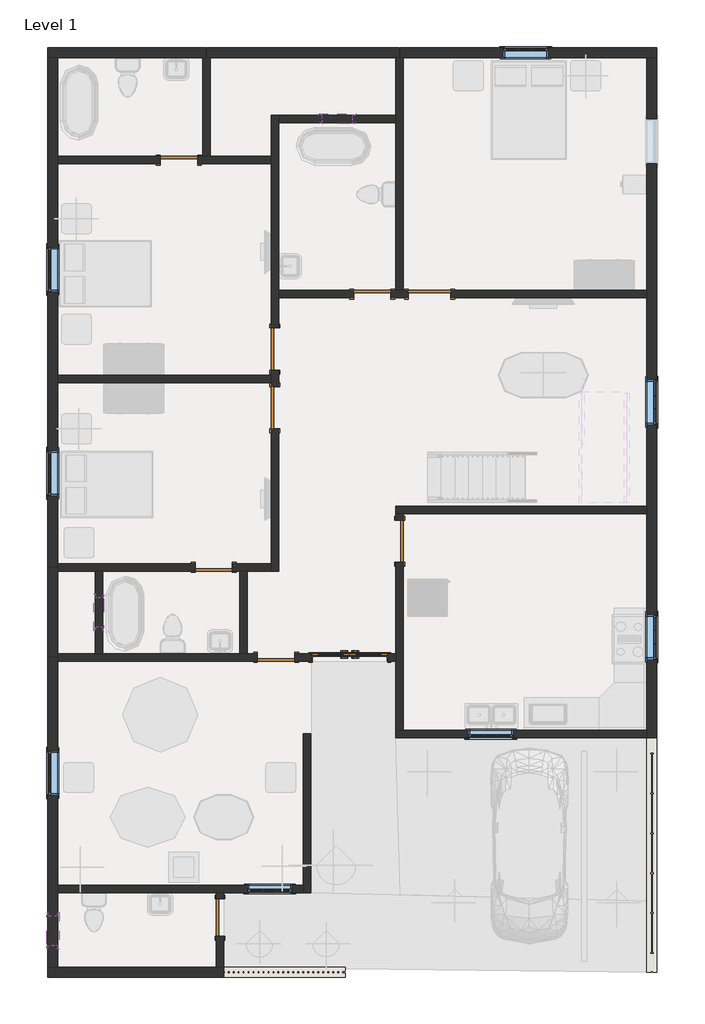
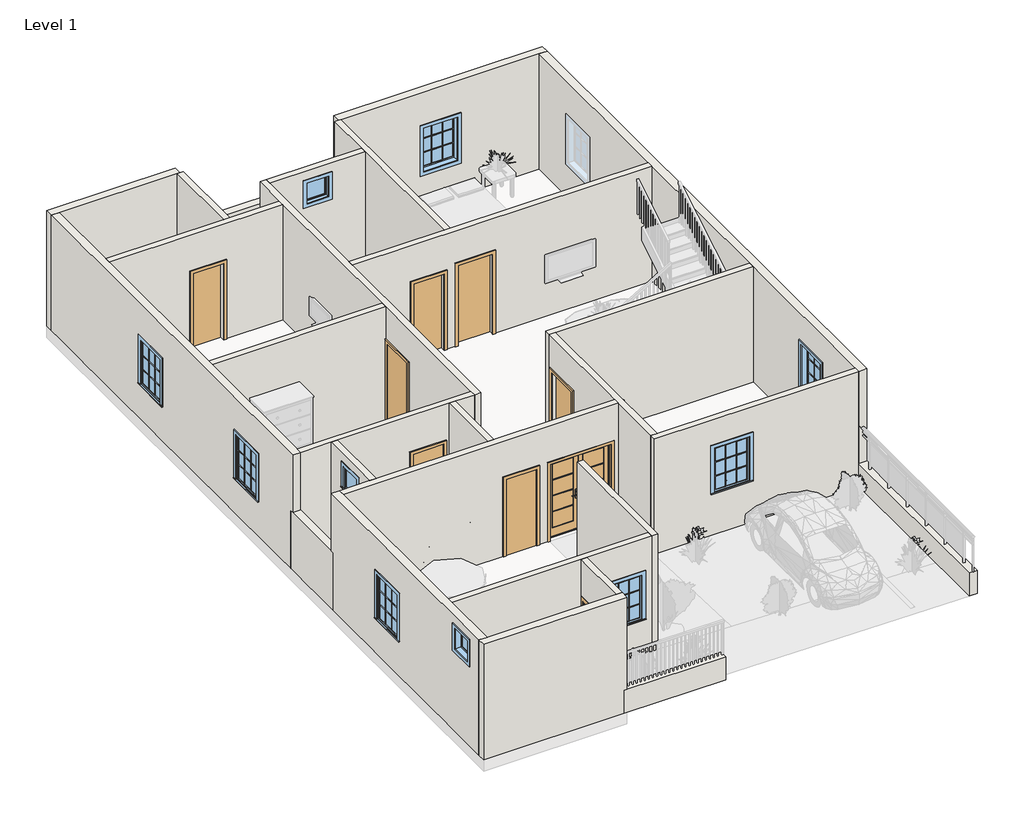
# One storey, part 1 of 3: 27 walls, 11 windows, 10 doors.
"""IFC4 building model written with IfcOpenShell, lengths in millimetres."""

from ifc_helpers import new_model, si_unit, frame, origin, origin_with_axes, place, context, project, spatial, polyline, outline, extrude, faceted_brep, transform, mapped, element, save
from components import door_94998e6c, door_255cab33, door_059fdd7e, door_99d96fc5, door_b6e9fca3, window_29c06734, window_5c190c7e, window_7947f0f9, window_e41d21a6, window_3d781103

model = new_model("IFC4")

# Units and contexts
model_context = context("Model", 3, world=origin())
ifc_project = project(units=[si_unit("LENGTHUNIT", "METRE", prefix="MILLI")], contexts=[model_context])

# Site, building, storey
site = spatial("IfcSite", under=ifc_project)
building = spatial("IfcBuilding", under=site)
storey = spatial("IfcBuildingStorey", under=building, Name="Level 1", Elevation=0.0)

# Doors
placement = place(None, origin())
door_shape = door_94998e6c(model_context)
element("IfcDoor", 1, ObjectType="Door-Exterior-Double-Full Glass-Wood_Clad : 60\" x 80\"", at=placement, inside=storey, context=model_context, shape_type="MappedRepresentation", body=[
    mapped(door_shape, transform((-5987.4789517, -1208.045591, 0.0), x_axis=(1.0, 0.0, 0.0), y_axis=(0.0, 1.0, 0.0), z_axis=(0.0, 0.0, 1.0))),
])
door_2_shape = door_255cab33(model_context)
element("IfcDoor", 2, ObjectType="Single-Flush : 30\" x 80\"", at=placement, inside=storey, context=model_context, shape_type="MappedRepresentation", body=[
    mapped(door_2_shape, transform((-8756.0789517, 617.579409, 0.0), x_axis=(1.0, 0.0, 0.0), y_axis=(0.0, 1.0, 0.0), z_axis=(0.0, 0.0, 1.0))),
])
element("IfcDoor", 3, ObjectType="Single-Flush : 30\" x 80\"", at=placement, inside=storey, context=model_context, shape_type="MappedRepresentation", body=[
    mapped(door_2_shape, transform((-7486.0789517, -1211.220591, 0.0), x_axis=(1.0, 0.0, 0.0), y_axis=(0.0, 1.0, 0.0), z_axis=(0.0, 0.0, 1.0))),
])
door_3_shape = door_059fdd7e(model_context)
element("IfcDoor", 4, ObjectType="Single-Flush : 30\" x 80\"", at=placement, inside=storey, context=model_context, shape_type="MappedRepresentation", body=[
    mapped(door_3_shape, transform((-9467.2789517, 8909.7768478, 0.0), x_axis=(1.0, 0.0, 0.0), y_axis=(0.0, 1.0, 0.0), z_axis=(0.0, 0.0, 1.0))),
])
element("IfcDoor", 5, ObjectType="Single-Flush : 30\" x 80\"", at=placement, inside=storey, context=model_context, shape_type="MappedRepresentation", body=[
    mapped(door_3_shape, transform((-5530.2789517, 6180.179409, 0.0), x_axis=(1.0, 0.0, 0.0), y_axis=(0.0, 1.0, 0.0), z_axis=(0.0, 0.0, 1.0))),
])
element("IfcDoor", 6, ObjectType="Single-Flush : 30\" x 80\"", at=placement, inside=storey, context=model_context, shape_type="MappedRepresentation", body=[
    mapped(door_3_shape, transform((-8629.0789517, -6508.0231522, 0.0), x_axis=(0.0, 1.0, 0.0), y_axis=(-1.0, 0.0, 0.0), z_axis=(0.0, 0.0, 1.0))),
])
door_4_shape = door_99d96fc5(model_context)
element("IfcDoor", 7, ObjectType="Single-Flush : 34\" x 84\"", at=placement, inside=storey, context=model_context, shape_type="MappedRepresentation", body=[
    mapped(door_4_shape, transform((-7511.4789517, 5062.579409, 0.0), x_axis=(0.0, -1.0, 0.0), y_axis=(1.0, 0.0, 0.0), z_axis=(0.0, 0.0, 1.0))),
])
element("IfcDoor", 8, ObjectType="Single-Flush : 34\" x 84\"", at=placement, inside=storey, context=model_context, shape_type="MappedRepresentation", body=[
    mapped(door_4_shape, transform((-4971.4789517, 1150.979409, 0.0), x_axis=(0.0, 1.0, 0.0), y_axis=(-1.0, 0.0, 0.0), z_axis=(0.0, 0.0, 1.0))),
])
element("IfcDoor", 9, ObjectType="Single-Flush : 34\" x 84\"", at=placement, inside=storey, context=model_context, shape_type="MappedRepresentation", body=[
    mapped(door_4_shape, transform((-4361.8789517, 6180.179409, 0.0), x_axis=(-1.0, 0.0, 0.0), y_axis=(0.0, -1.0, 0.0), z_axis=(0.0, 0.0, 1.0))),
])
door_5_shape = door_b6e9fca3(model_context)
element("IfcDoor", 10, ObjectType="Single-Flush : 34\" x 84\"", at=placement, inside=storey, context=model_context, shape_type="MappedRepresentation", body=[
    mapped(door_5_shape, transform((-7511.4789517, 3868.779409, 0.0), x_axis=(0.0, 1.0, 0.0), y_axis=(-1.0, 0.0, 0.0), z_axis=(0.0, 0.0, 1.0))),
])

# Walls
element("IfcWall", 11, ObjectType="Generic - 2'", at=placement, inside=storey, context=model_context, shape_type="Brep", body=[
    faceted_brep([(-6079.5539517, -7524.0231522, 0.0), (-8552.8789517, -7524.0231522, 0.0), (-8629.0789517, -7524.0231522, 0.0), (-8629.0789517, -7524.0231522, 609.6), (-6079.5539517, -7524.0231522, 609.6), (-6079.5539517, -7727.2231522, 0.0), (-6079.5539517, -7727.2231522, 609.6), (-8629.0789517, -7727.2231522, 609.6), (-8629.0789517, -7727.2231522, 0.0)], [[[0, 1, 2, 3, 4]], [[5, 6, 7, 8]], [[2, 1, 0, 5, 8]], [[3, 2, 8, 7]], [[4, 3, 7, 6]], [[0, 4, 6, 5]]]),
])
element("IfcWall", 12, ObjectType="Generic - 2'", at=placement, inside=storey, context=model_context, shape_type="Brep", body=[
    faceted_brep([(57.7210483, -2774.2231522, 0.0), (57.7210483, -2850.4231522, 0.0), (57.7210483, -7625.6231522, 0.0), (57.7210483, -7625.6231522, 609.6), (57.7210483, -2774.2231522, 609.6), (260.9210483, -2774.2231522, 0.0), (260.9210483, -2774.2231522, 609.6), (260.9210483, -7625.6231522, 609.6), (260.9210483, -7625.6231522, 0.0)], [[[0, 1, 2, 3, 4]], [[5, 6, 7, 8]], [[2, 1, 0, 5, 8]], [[3, 2, 8, 7]], [[4, 3, 7, 6]], [[0, 4, 6, 5]]]),
])
element("IfcWall", 13, ObjectType="Generic - 8\"", at=placement, inside=storey, context=model_context, shape_type="Brep", body=[
    faceted_brep([(-12134.2789517, 10992.5768478, 0.0), (-11931.0789517, 10992.5768478, 0.0), (-8921.1789517, 10992.5768478, 0.0), (-8921.1789517, 10992.5768478, 3048.0), (-11931.0789517, 10992.5768478, 3048.0), (-12134.2789517, 10992.5768478, 3048.0), (-12134.2789517, 11195.7768478, 0.0), (-12134.2789517, 11195.7768478, 3048.0), (-8921.1789517, 11195.7768478, 3048.0), (-8921.1789517, 11195.7768478, 0.0)], [[[0, 1, 2, 3, 4, 5]], [[6, 7, 8, 9]], [[2, 1, 0, 6, 9]], [[3, 2, 9, 8]], [[0, 5, 7, 6]], [[5, 4, 3, 8, 7]]]),
])
element("IfcWall", 14, ObjectType="Generic - 8\"", at=placement, inside=storey, context=model_context, shape_type="Brep", body=[
    faceted_brep([(57.7210483, 10992.5768478, 0.0), (57.7210483, 6256.379409, 0.0), (57.7210483, 6103.979409, 0.0), (57.7210483, 1862.179409, 0.0), (57.7210483, 1709.779409, 0.0), (57.7210483, -2698.0231522, 0.0), (57.7210483, -2774.2231522, 0.0), (57.7210483, -2774.2231522, 609.6), (57.7210483, -2850.4231522, 609.6), (57.7210483, -2850.4231522, 3048.0), (57.7210483, -2698.0231522, 3048.0), (57.7210483, 1709.779409, 3048.0), (57.7210483, 1862.179409, 3048.0), (57.7210483, 6103.979409, 3048.0), (57.7210483, 6256.379409, 3048.0), (57.7210483, 10992.5768478, 3048.0), (57.7210483, -1256.1218716, 2286.0), (57.7210483, -1256.1218716, 1066.8), (57.7210483, -341.7218716, 1066.8), (57.7210483, -341.7218716, 2286.0), (57.7210483, 3525.879409, 2133.6), (57.7210483, 3525.879409, 914.4), (57.7210483, 4440.279409, 914.4), (57.7210483, 4440.279409, 2133.6), (57.7210483, 8833.5768478, 2133.6), (57.7210483, 8833.5768478, 914.4), (57.7210483, 9747.9768478, 914.4), (57.7210483, 9747.9768478, 2133.6), (260.9210483, 10992.5768478, 0.0), (260.9210483, 10992.5768478, 3048.0), (260.9210483, -2850.4231522, 3048.0), (260.9210483, -2850.4231522, 609.6), (260.9210483, -2774.2231522, 609.6), (260.9210483, -2774.2231522, 0.0), (260.9210483, -1256.1218716, 2286.0), (260.9210483, -341.7218716, 2286.0), (260.9210483, -341.7218716, 1066.8), (260.9210483, -1256.1218716, 1066.8), (260.9210483, 3525.879409, 2133.6), (260.9210483, 4440.279409, 2133.6), (260.9210483, 4440.279409, 914.4), (260.9210483, 3525.879409, 914.4), (260.9210483, 8833.5768478, 2133.6), (260.9210483, 9747.9768478, 2133.6), (260.9210483, 9747.9768478, 914.4), (260.9210483, 8833.5768478, 914.4)], [[[0, 1, 2, 3, 4, 5, 6, 7, 8, 9, 10, 11, 12, 13, 14, 15], [16, 17, 18, 19], [20, 21, 22, 23], [24, 25, 26, 27]], [[28, 29, 30, 31, 32, 33], [34, 35, 36, 37], [38, 39, 40, 41], [42, 43, 44, 45]], [[6, 5, 4, 3, 2, 1, 0, 28, 33]], [[0, 15, 29, 28]], [[17, 16, 34, 37]], [[18, 17, 37, 36]], [[19, 18, 36, 35]], [[16, 19, 35, 34]], [[21, 20, 38, 41]], [[22, 21, 41, 40]], [[23, 22, 40, 39]], [[20, 23, 39, 38]], [[25, 24, 42, 45]], [[26, 25, 45, 44]], [[27, 26, 44, 43]], [[24, 27, 43, 42]], [[7, 6, 33, 32]], [[31, 8, 7, 32]], [[9, 8, 31, 30]], [[15, 14, 13, 12, 11, 10, 9, 30, 29]]]),
])
element("IfcWall", 15, ObjectType="Generic - 8\"", at=placement, inside=storey, context=model_context, shape_type="Brep", body=[
    faceted_brep([(-11931.0789517, -7524.0231522, 0.0), (-11931.0789517, -6000.0231522, 0.0), (-11931.0789517, -5847.6231522, 0.0), (-11931.0789517, -1287.420591, 0.0), (-11931.0789517, -1211.220591, 0.0), (-11931.0789517, -1211.220591, 1524.0), (-11931.0789517, -1135.020591, 1524.0), (-11931.0789517, -1135.020591, 3048.0), (-11931.0789517, -1287.420591, 3048.0), (-11931.0789517, -5847.6231522, 3048.0), (-11931.0789517, -6000.0231522, 3048.0), (-11931.0789517, -7524.0231522, 3048.0), (-11931.0789517, -3110.3218716, 2133.6), (-11931.0789517, -3110.3218716, 914.4), (-11931.0789517, -4024.7218716, 914.4), (-11931.0789517, -4024.7218716, 2133.6), (-11931.0789517, -7079.5231522, 2768.6), (-11931.0789517, -6469.9231522, 2768.6), (-11931.0789517, -6469.9231522, 2159.0), (-11931.0789517, -7079.5231522, 2159.0), (-12134.2789517, -7524.0231522, 0.0), (-12134.2789517, -7524.0231522, 3048.0), (-12134.2789517, -1135.020591, 3048.0), (-12134.2789517, -1135.020591, 1524.0), (-12134.2789517, -1211.220591, 1524.0), (-12134.2789517, -1211.220591, 0.0), (-12134.2789517, -3110.3218716, 2133.6), (-12134.2789517, -4024.7218716, 2133.6), (-12134.2789517, -4024.7218716, 914.4), (-12134.2789517, -3110.3218716, 914.4), (-12134.2789517, -7079.5231522, 2768.6), (-12134.2789517, -7079.5231522, 2159.0), (-12134.2789517, -6469.9231522, 2159.0), (-12134.2789517, -6469.9231522, 2768.6)], [[[0, 1, 2, 3, 4, 5, 6, 7, 8, 9, 10, 11], [12, 13, 14, 15], [16, 17, 18, 19]], [[20, 21, 22, 23, 24, 25], [26, 27, 28, 29], [30, 31, 32, 33]], [[4, 3, 2, 1, 0, 20, 25]], [[0, 11, 21, 20]], [[13, 12, 26, 29]], [[14, 13, 29, 28]], [[15, 14, 28, 27]], [[12, 15, 27, 26]], [[31, 30, 16, 19]], [[32, 31, 19, 18]], [[33, 32, 18, 17]], [[30, 33, 17, 16]], [[5, 4, 25, 24]], [[23, 6, 5, 24]], [[7, 6, 23, 22]], [[11, 10, 9, 8, 7, 22, 21]]]),
])
element("IfcWall", 16, ObjectType="Generic - 8\"", at=placement, inside=storey, context=model_context, shape_type="Brep", body=[
    faceted_brep([(-8629.0789517, -7524.0231522, 0.0), (-8705.2789517, -7524.0231522, 0.0), (-11931.0789517, -7524.0231522, 0.0), (-12134.2789517, -7524.0231522, 0.0), (-12134.2789517, -7524.0231522, 3048.0), (-11931.0789517, -7524.0231522, 3048.0), (-8705.2789517, -7524.0231522, 3048.0), (-8552.8789517, -7524.0231522, 3048.0), (-8552.8789517, -7524.0231522, 609.6), (-8629.0789517, -7524.0231522, 609.6), (-8629.0789517, -7727.2231522, 0.0), (-8629.0789517, -7727.2231522, 609.6), (-8552.8789517, -7727.2231522, 609.6), (-8552.8789517, -7727.2231522, 3048.0), (-12134.2789517, -7727.2231522, 3048.0), (-12134.2789517, -7727.2231522, 0.0)], [[[0, 1, 2, 3, 4, 5, 6, 7, 8, 9]], [[10, 11, 12, 13, 14, 15]], [[3, 2, 1, 0, 10, 15]], [[4, 3, 15, 14]], [[0, 9, 11, 10]], [[8, 12, 11, 9]], [[8, 7, 13, 12]], [[7, 6, 5, 4, 14, 13]]]),
])
element("IfcWall", 17, ObjectType="Generic - 8\"", at=placement, inside=storey, context=model_context, shape_type="Brep", body=[
    faceted_brep([(-8895.7789517, 10992.5768478, 0.0), (-8832.2789517, 10992.5768478, 0.0), (-4984.1789517, 10992.5768478, 0.0), (-4984.1789517, 10992.5768478, 1524.0), (-8895.7789517, 10992.5768478, 1524.0), (-8895.7789517, 11195.7768478, 0.0), (-8895.7789517, 11195.7768478, 1524.0), (-4984.1789517, 11195.7768478, 1524.0), (-4984.1789517, 11195.7768478, 0.0)], [[[0, 1, 2, 3, 4]], [[5, 6, 7, 8]], [[2, 1, 0, 5, 8]], [[3, 2, 8, 7]], [[4, 3, 7, 6]], [[0, 4, 6, 5]]]),
])
element("IfcWall", 18, ObjectType="Generic - 8\"", at=placement, inside=storey, context=model_context, shape_type="Brep", body=[
    faceted_brep([(-4958.7789517, 10992.5768478, 0.0), (-4895.2789517, 10992.5768478, 0.0), (57.7210483, 10992.5768478, 0.0), (260.9210483, 10992.5768478, 0.0), (260.9210483, 10992.5768478, 3048.0), (57.7210483, 10992.5768478, 3048.0), (-4895.2789517, 10992.5768478, 3048.0), (-4958.7789517, 10992.5768478, 3048.0), (-1948.8789517, 10992.5768478, 2133.6), (-1948.8789517, 10992.5768478, 914.4), (-2863.2789517, 10992.5768478, 914.4), (-2863.2789517, 10992.5768478, 2133.6), (-4958.7789517, 11195.7768478, 0.0), (-4958.7789517, 11195.7768478, 3048.0), (260.9210483, 11195.7768478, 3048.0), (260.9210483, 11195.7768478, 0.0), (-1948.8789517, 11195.7768478, 2133.6), (-2863.2789517, 11195.7768478, 2133.6), (-2863.2789517, 11195.7768478, 914.4), (-1948.8789517, 11195.7768478, 914.4)], [[[0, 1, 2, 3, 4, 5, 6, 7], [8, 9, 10, 11]], [[12, 13, 14, 15], [16, 17, 18, 19]], [[3, 2, 1, 0, 12, 15]], [[0, 7, 13, 12]], [[4, 3, 15, 14]], [[8, 11, 17, 16]], [[11, 10, 18, 17]], [[10, 9, 19, 18]], [[9, 8, 16, 19]], [[7, 6, 5, 4, 14, 13]]]),
])
element("IfcWall", 19, ObjectType="Generic - 8\"", at=placement, inside=storey, context=model_context, shape_type="Brep", body=[
    faceted_brep([(-11931.0789517, 617.579409, 0.0), (-11931.0789517, 693.779409, 0.0), (-11931.0789517, 4376.779409, 0.0), (-11931.0789517, 4529.179409, 0.0), (-11931.0789517, 8833.5768478, 0.0), (-11931.0789517, 8985.9768478, 0.0), (-11931.0789517, 10992.5768478, 0.0), (-11931.0789517, 10992.5768478, 3048.0), (-11931.0789517, 8985.9768478, 3048.0), (-11931.0789517, 8833.5768478, 3048.0), (-11931.0789517, 4529.179409, 3048.0), (-11931.0789517, 4376.779409, 3048.0), (-11931.0789517, 693.779409, 3048.0), (-11931.0789517, 541.379409, 3048.0), (-11931.0789517, 541.379409, 1524.0), (-11931.0789517, 617.579409, 1524.0), (-11931.0789517, 7138.5781284, 2133.6), (-11931.0789517, 7138.5781284, 914.4), (-11931.0789517, 6224.1781284, 914.4), (-11931.0789517, 6224.1781284, 2133.6), (-11931.0789517, 2992.479409, 2133.6), (-11931.0789517, 2992.479409, 914.4), (-11931.0789517, 2078.079409, 914.4), (-11931.0789517, 2078.079409, 2133.6), (-12134.2789517, 617.579409, 0.0), (-12134.2789517, 617.579409, 1524.0), (-12134.2789517, 541.379409, 1524.0), (-12134.2789517, 541.379409, 3048.0), (-12134.2789517, 10992.5768478, 3048.0), (-12134.2789517, 10992.5768478, 0.0), (-12134.2789517, 7138.5781284, 2133.6), (-12134.2789517, 6224.1781284, 2133.6), (-12134.2789517, 6224.1781284, 914.4), (-12134.2789517, 7138.5781284, 914.4), (-12134.2789517, 2992.479409, 2133.6), (-12134.2789517, 2078.079409, 2133.6), (-12134.2789517, 2078.079409, 914.4), (-12134.2789517, 2992.479409, 914.4)], [[[0, 1, 2, 3, 4, 5, 6, 7, 8, 9, 10, 11, 12, 13, 14, 15], [16, 17, 18, 19], [20, 21, 22, 23]], [[24, 25, 26, 27, 28, 29], [30, 31, 32, 33], [34, 35, 36, 37]], [[6, 5, 4, 3, 2, 1, 0, 24, 29]], [[7, 6, 29, 28]], [[16, 19, 31, 30]], [[19, 18, 32, 31]], [[18, 17, 33, 32]], [[17, 16, 30, 33]], [[20, 23, 35, 34]], [[23, 22, 36, 35]], [[22, 21, 37, 36]], [[21, 20, 34, 37]], [[0, 15, 25, 24]], [[14, 26, 25, 15]], [[14, 13, 27, 26]], [[13, 12, 11, 10, 9, 8, 7, 28, 27]]]),
])
element("IfcWall", 20, ObjectType="Generic - 8\"", at=placement, inside=storey, context=model_context, shape_type="Brep", body=[
    faceted_brep([(-11931.0789517, -1211.220591, 0.0), (-11931.0789517, -1135.020591, 0.0), (-11931.0789517, 541.379409, 0.0), (-11931.0789517, 617.579409, 0.0), (-11931.0789517, 617.579409, 1524.0), (-11931.0789517, 541.379409, 1524.0), (-11931.0789517, -1135.020591, 1524.0), (-11931.0789517, -1211.220591, 1524.0), (-12134.2789517, -1211.220591, 0.0), (-12134.2789517, -1211.220591, 1524.0), (-12134.2789517, -1135.020591, 1524.0), (-12134.2789517, 541.379409, 1524.0), (-12134.2789517, 617.579409, 1524.0), (-12134.2789517, 617.579409, 0.0)], [[[0, 1, 2, 3, 4, 5, 6, 7]], [[8, 9, 10, 11, 12, 13]], [[3, 2, 1, 0, 8, 13]], [[4, 3, 13, 12]], [[7, 6, 5, 4, 12, 11, 10, 9]], [[0, 7, 9, 8]]]),
])
element("IfcWall", 21, ObjectType="INNER 6\"", at=placement, inside=storey, context=model_context, shape_type="Brep", body=[
    faceted_brep([(-9086.2789517, 8833.5768478, 2032.0), (-9086.2789517, 8833.5768478, 0.0), (-7587.6789517, 8833.5768478, 0.0), (-7587.6789517, 8833.5768478, 3048.0), (-11931.0789517, 8833.5768478, 3048.0), (-11931.0789517, 8833.5768478, 0.0), (-9848.2789517, 8833.5768478, 0.0), (-9848.2789517, 8833.5768478, 2032.0), (-7587.6789517, 8985.9768478, 0.0), (-8832.2789517, 8985.9768478, 0.0), (-8984.6789517, 8985.9768478, 0.0), (-9086.2789517, 8985.9768478, 0.0), (-9086.2789517, 8985.9768478, 2032.0), (-9848.2789517, 8985.9768478, 2032.0), (-9848.2789517, 8985.9768478, 0.0), (-11931.0789517, 8985.9768478, 0.0), (-11931.0789517, 8985.9768478, 3048.0), (-8984.6789517, 8985.9768478, 3048.0), (-8832.2789517, 8985.9768478, 3048.0), (-7587.6789517, 8985.9768478, 3048.0)], [[[0, 1, 2, 3, 4, 5, 6, 7]], [[8, 9, 10, 11, 12, 13, 14, 15, 16, 17, 18, 19]], [[6, 5, 15, 14]], [[2, 1, 11, 10, 9, 8]], [[5, 4, 16, 15]], [[3, 2, 8, 19]], [[12, 11, 1, 0]], [[13, 12, 0, 7]], [[14, 13, 7, 6]], [[4, 3, 19, 18, 17, 16]]]),
])
element("IfcWall", 22, ObjectType="INNER 6\"", at=placement, inside=storey, context=model_context, shape_type="Brep", body=[
    faceted_brep([(-8832.2789517, 8985.9768478, 0.0), (-8832.2789517, 10992.5768478, 0.0), (-8832.2789517, 10992.5768478, 3048.0), (-8832.2789517, 8985.9768478, 3048.0), (-8984.6789517, 8985.9768478, 0.0), (-8984.6789517, 8985.9768478, 3048.0), (-8984.6789517, 10992.5768478, 3048.0), (-8984.6789517, 10992.5768478, 0.0), (-8895.7789517, 10992.5768478, 0.0)], [[[0, 1, 2, 3]], [[4, 5, 6, 7]], [[1, 0, 4, 7, 8]], [[0, 3, 5, 4]], [[2, 1, 8, 7, 6]], [[3, 2, 6, 5]]]),
])
element("IfcWall", 23, ObjectType="INNER 6\"", at=placement, inside=storey, context=model_context, shape_type="Brep", body=[
    faceted_brep([(-7435.2789517, 4300.579409, 2133.6), (-7435.2789517, 4300.579409, 0.0), (-7435.2789517, 4630.779409, 0.0), (-7435.2789517, 4630.779409, 2133.6), (-7435.2789517, 5494.379409, 2133.6), (-7435.2789517, 5494.379409, 0.0), (-7435.2789517, 6103.979409, 0.0), (-7435.2789517, 6256.379409, 0.0), (-7435.2789517, 9671.7768478, 0.0), (-7435.2789517, 9824.1768478, 0.0), (-7435.2789517, 9824.1768478, 3048.0), (-7435.2789517, 9671.7768478, 3048.0), (-7435.2789517, 6256.379409, 3048.0), (-7435.2789517, 6103.979409, 3048.0), (-7435.2789517, 541.379409, 3048.0), (-7435.2789517, 541.379409, 0.0), (-7435.2789517, 3436.979409, 0.0), (-7435.2789517, 3436.979409, 2133.6), (-7587.6789517, 4630.779409, 0.0), (-7587.6789517, 4529.179409, 0.0), (-7587.6789517, 4376.779409, 0.0), (-7587.6789517, 4300.579409, 0.0), (-7587.6789517, 4300.579409, 2133.6), (-7587.6789517, 3436.979409, 2133.6), (-7587.6789517, 3436.979409, 0.0), (-7587.6789517, 693.779409, 0.0), (-7587.6789517, 541.379409, 0.0), (-7587.6789517, 541.379409, 3048.0), (-7587.6789517, 693.779409, 3048.0), (-7587.6789517, 4376.779409, 3048.0), (-7587.6789517, 4529.179409, 3048.0), (-7587.6789517, 8833.5768478, 3048.0), (-7587.6789517, 8985.9768478, 3048.0), (-7587.6789517, 9824.1768478, 3048.0), (-7587.6789517, 9824.1768478, 0.0), (-7587.6789517, 8985.9768478, 0.0), (-7587.6789517, 8833.5768478, 0.0), (-7587.6789517, 5494.379409, 0.0), (-7587.6789517, 5494.379409, 2133.6), (-7587.6789517, 4630.779409, 2133.6)], [[[0, 1, 2, 3, 4, 5, 6, 7, 8, 9, 10, 11, 12, 13, 14, 15, 16, 17]], [[18, 19, 20, 21, 22, 23, 24, 25, 26, 27, 28, 29, 30, 31, 32, 33, 34, 35, 36, 37, 38, 39]], [[37, 36, 35, 34, 9, 8, 7, 6, 5]], [[16, 15, 26, 25, 24]], [[2, 1, 21, 20, 19, 18]], [[10, 9, 34, 33]], [[15, 14, 27, 26]], [[3, 2, 18, 39]], [[4, 3, 39, 38]], [[5, 4, 38, 37]], [[22, 21, 1, 0]], [[23, 22, 0, 17]], [[24, 23, 17, 16]], [[14, 13, 12, 11, 10, 33, 32, 31, 30, 29, 28, 27]]]),
])
element("IfcWall", 24, ObjectType="INNER 6\"", at=placement, inside=storey, context=model_context, shape_type="SweptSolid", body=[
    extrude(outline(polyline([(0.0, -7435.2789517), (0.0, -5047.6789517), (3048.0, -5047.6789517), (3048.0, -7435.2789517), (0.0, -7435.2789517)]), holes=[polyline([(2768.6, -5936.6789517), (2159.0, -5936.6789517), (2159.0, -6546.2789517), (2768.6, -6546.2789517), (2768.6, -5936.6789517)])]), frame((0.0, 9671.7768478, 0.0), z_axis=(0.0, 1.0, 0.0), x_axis=(0.0, 0.0, 1.0)), (0.0, 0.0, 1.0), 152.4),
])
element("IfcWall", 25, ObjectType="INNER 6\"", at=placement, inside=storey, context=model_context, shape_type="Brep", body=[
    faceted_brep([(-5047.6789517, 10992.5768478, 0.0), (-5047.6789517, 9824.1768478, 0.0), (-5047.6789517, 9671.7768478, 0.0), (-5047.6789517, 6256.379409, 0.0), (-5047.6789517, 6256.379409, 3048.0), (-5047.6789517, 9671.7768478, 3048.0), (-5047.6789517, 9824.1768478, 3048.0), (-5047.6789517, 10992.5768478, 3048.0), (-4895.2789517, 10992.5768478, 0.0), (-4895.2789517, 10992.5768478, 3048.0), (-4895.2789517, 6256.379409, 3048.0), (-4895.2789517, 6256.379409, 0.0), (-4958.7789517, 10992.5768478, 0.0), (-4958.7789517, 10992.5768478, 3048.0)], [[[0, 1, 2, 3, 4, 5, 6, 7]], [[8, 9, 10, 11]], [[3, 2, 1, 0, 12, 8, 11]], [[0, 7, 13, 9, 8, 12]], [[4, 3, 11, 10]], [[7, 6, 5, 4, 10, 9, 13]]]),
])
element("IfcWall", 26, ObjectType="INNER 6\"", at=placement, inside=storey, context=model_context, shape_type="Brep", body=[
    faceted_brep([(-5149.2789517, 6103.979409, 2032.0), (-5149.2789517, 6103.979409, 0.0), (-4793.6789517, 6103.979409, 0.0), (-4793.6789517, 6103.979409, 2133.6), (-3930.0789517, 6103.979409, 2133.6), (-3930.0789517, 6103.979409, 0.0), (57.7210483, 6103.979409, 0.0), (57.7210483, 6103.979409, 3048.0), (-7435.2789517, 6103.979409, 3048.0), (-7435.2789517, 6103.979409, 0.0), (-5911.2789517, 6103.979409, 0.0), (-5911.2789517, 6103.979409, 2032.0), (-4793.6789517, 6256.379409, 0.0), (-4895.2789517, 6256.379409, 0.0), (-5047.6789517, 6256.379409, 0.0), (-5149.2789517, 6256.379409, 0.0), (-5149.2789517, 6256.379409, 2032.0), (-5911.2789517, 6256.379409, 2032.0), (-5911.2789517, 6256.379409, 0.0), (-7435.2789517, 6256.379409, 0.0), (-7435.2789517, 6256.379409, 3048.0), (-5047.6789517, 6256.379409, 3048.0), (-4895.2789517, 6256.379409, 3048.0), (57.7210483, 6256.379409, 3048.0), (57.7210483, 6256.379409, 0.0), (-3930.0789517, 6256.379409, 0.0), (-3930.0789517, 6256.379409, 2133.6), (-4793.6789517, 6256.379409, 2133.6)], [[[0, 1, 2, 3, 4, 5, 6, 7, 8, 9, 10, 11]], [[12, 13, 14, 15, 16, 17, 18, 19, 20, 21, 22, 23, 24, 25, 26, 27]], [[25, 24, 6, 5]], [[10, 9, 19, 18]], [[2, 1, 15, 14, 13, 12]], [[7, 6, 24, 23]], [[9, 8, 20, 19]], [[3, 2, 12, 27]], [[4, 3, 27, 26]], [[5, 4, 26, 25]], [[16, 15, 1, 0]], [[17, 16, 0, 11]], [[18, 17, 11, 10]], [[8, 7, 23, 22, 21, 20]]]),
])
element("IfcWall", 27, ObjectType="INNER 6\"", at=placement, inside=storey, context=model_context, shape_type="Brep", body=[
    faceted_brep([(-5047.6789517, 1709.779409, 0.0), (-4895.2789517, 1709.779409, 0.0), (57.7210483, 1709.779409, 0.0), (57.7210483, 1709.779409, 3048.0), (-4895.2789517, 1709.779409, 3048.0), (-5047.6789517, 1709.779409, 3048.0), (-5047.6789517, 1862.179409, 0.0), (-5047.6789517, 1862.179409, 3048.0), (57.7210483, 1862.179409, 3048.0), (57.7210483, 1862.179409, 0.0)], [[[0, 1, 2, 3, 4, 5]], [[6, 7, 8, 9]], [[2, 1, 0, 6, 9]], [[3, 2, 9, 8]], [[0, 5, 7, 6]], [[5, 4, 3, 8, 7]]]),
])
element("IfcWall", 28, ObjectType="INNER 6\"", at=placement, inside=storey, context=model_context, shape_type="Brep", body=[
    faceted_brep([(-5047.6789517, -2850.4231522, 0.0), (57.7210483, -2850.4231522, 0.0), (57.7210483, -2850.4231522, 609.6), (57.7210483, -2850.4231522, 3048.0), (-5047.6789517, -2850.4231522, 3048.0), (-3574.4789517, -2850.4231522, 2311.4), (-2660.0789517, -2850.4231522, 2311.4), (-2660.0789517, -2850.4231522, 1092.2), (-3574.4789517, -2850.4231522, 1092.2), (-5047.6789517, -2698.0231522, 0.0), (-5047.6789517, -2698.0231522, 3048.0), (-4895.2789517, -2698.0231522, 3048.0), (57.7210483, -2698.0231522, 3048.0), (57.7210483, -2698.0231522, 0.0), (-4895.2789517, -2698.0231522, 0.0), (-3574.4789517, -2698.0231522, 2311.4), (-3574.4789517, -2698.0231522, 1092.2), (-2660.0789517, -2698.0231522, 1092.2), (-2660.0789517, -2698.0231522, 2311.4), (57.7210483, -2774.2231522, 0.0)], [[[0, 1, 2, 3, 4], [5, 6, 7, 8]], [[9, 10, 11, 12, 13, 14], [15, 16, 17, 18]], [[1, 0, 9, 14, 13, 19]], [[0, 4, 10, 9]], [[16, 15, 5, 8]], [[17, 16, 8, 7]], [[18, 17, 7, 6]], [[15, 18, 6, 5]], [[1, 19, 13, 12, 3, 2]], [[4, 3, 12, 11, 10]]]),
])
element("IfcWall", 29, ObjectType="INNER 6\"", at=placement, inside=storey, context=model_context, shape_type="SweptSolid", body=[
    extrude(outline(polyline([(-7587.6789517, 4376.779409), (-11931.0789517, 4376.779409), (-11931.0789517, 4529.179409), (-7587.6789517, 4529.179409), (-7587.6789517, 4376.779409)])), origin_with_axes(), (0.0, 0.0, 1.0), 3048.0),
])
element("IfcWall", 30, ObjectType="INNER 6\"", at=placement, inside=storey, context=model_context, shape_type="Brep", body=[
    faceted_brep([(-7587.6789517, 693.779409, 0.0), (-8375.0789517, 693.779409, 0.0), (-8375.0789517, 693.779409, 2032.0), (-9137.0789517, 693.779409, 2032.0), (-9137.0789517, 693.779409, 0.0), (-11931.0789517, 693.779409, 0.0), (-11931.0789517, 693.779409, 3048.0), (-7587.6789517, 693.779409, 3048.0), (-8375.0789517, 541.379409, 2032.0), (-8375.0789517, 541.379409, 0.0), (-8222.6789517, 541.379409, 0.0), (-8070.2789517, 541.379409, 0.0), (-7587.6789517, 541.379409, 0.0), (-7587.6789517, 541.379409, 3048.0), (-8070.2789517, 541.379409, 3048.0), (-8222.6789517, 541.379409, 3048.0), (-11016.6789517, 541.379409, 3048.0), (-11169.0789517, 541.379409, 3048.0), (-11931.0789517, 541.379409, 3048.0), (-11931.0789517, 541.379409, 1524.0), (-11931.0789517, 541.379409, 0.0), (-11169.0789517, 541.379409, 0.0), (-11016.6789517, 541.379409, 0.0), (-9137.0789517, 541.379409, 0.0), (-9137.0789517, 541.379409, 2032.0), (-11931.0789517, 617.579409, 0.0)], [[[0, 1, 2, 3, 4, 5, 6, 7]], [[8, 9, 10, 11, 12, 13, 14, 15, 16, 17, 18, 19, 20, 21, 22, 23, 24]], [[12, 11, 10, 9, 1, 0]], [[23, 22, 21, 20, 25, 5, 4]], [[0, 7, 13, 12]], [[2, 1, 9, 8]], [[3, 2, 8, 24]], [[4, 3, 24, 23]], [[5, 25, 20, 19, 18, 6]], [[7, 6, 18, 17, 16, 15, 14, 13]]]),
])
element("IfcWall", 31, ObjectType="INNER 6\"", at=placement, inside=storey, context=model_context, shape_type="SweptSolid", body=[
    extrude(outline(polyline([(-8222.6789517, -1135.020591), (-8222.6789517, 541.379409), (-8070.2789517, 541.379409), (-8070.2789517, -1135.020591), (-8222.6789517, -1135.020591)])), origin_with_axes(), (0.0, 0.0, 1.0), 3048.0),
])
element("IfcWall", 32, ObjectType="INNER 6\"", at=placement, inside=storey, context=model_context, shape_type="Brep", body=[
    faceted_brep([(-5047.6789517, -1135.020591, 3048.0), (-5047.6789517, -1135.020591, 0.0), (-5200.0789517, -1135.020591, 0.0), (-5200.0789517, -1135.020591, 2057.4), (-6774.8789517, -1135.020591, 2057.4), (-6774.8789517, -1135.020591, 0.0), (-7105.0789517, -1135.020591, 0.0), (-7105.0789517, -1135.020591, 2032.0), (-7867.0789517, -1135.020591, 2032.0), (-7867.0789517, -1135.020591, 0.0), (-8070.2789517, -1135.020591, 0.0), (-8222.6789517, -1135.020591, 0.0), (-11016.6789517, -1135.020591, 0.0), (-11169.0789517, -1135.020591, 0.0), (-11931.0789517, -1135.020591, 0.0), (-11931.0789517, -1135.020591, 1524.0), (-11931.0789517, -1135.020591, 3048.0), (-11169.0789517, -1135.020591, 3048.0), (-11016.6789517, -1135.020591, 3048.0), (-8222.6789517, -1135.020591, 3048.0), (-8070.2789517, -1135.020591, 3048.0), (-5047.6789517, -1287.420591, 0.0), (-5047.6789517, -1287.420591, 3048.0), (-6774.8789517, -1287.420591, 3048.0), (-11931.0789517, -1287.420591, 3048.0), (-11931.0789517, -1287.420591, 0.0), (-7867.0789517, -1287.420591, 0.0), (-7867.0789517, -1287.420591, 2032.0), (-7105.0789517, -1287.420591, 2032.0), (-7105.0789517, -1287.420591, 0.0), (-6774.8789517, -1287.420591, 0.0), (-6774.8789517, -1287.420591, 2057.4), (-5200.0789517, -1287.420591, 2057.4), (-5200.0789517, -1287.420591, 0.0), (-11931.0789517, -1211.220591, 0.0)], [[[0, 1, 2, 3, 4, 5, 6, 7, 8, 9, 10, 11, 12, 13, 14, 15, 16, 17, 18, 19, 20]], [[21, 22, 23, 24, 25, 26, 27, 28, 29, 30, 31, 32, 33]], [[1, 21, 33, 2]], [[29, 6, 5, 30]], [[25, 34, 14, 13, 12, 11, 10, 9, 26]], [[1, 0, 22, 21]], [[7, 6, 29, 28]], [[8, 7, 28, 27]], [[9, 8, 27, 26]], [[32, 3, 2, 33]], [[3, 32, 31, 4]], [[4, 31, 30, 5]], [[14, 34, 25, 24, 16, 15]], [[22, 0, 20, 19, 18, 17, 16, 24, 23]]]),
])
element("IfcWall", 33, ObjectType="INNER 6\"", at=placement, inside=storey, context=model_context, shape_type="Brep", body=[
    faceted_brep([(-5047.6789517, 1709.779409, 0.0), (-5047.6789517, 1582.779409, 0.0), (-5047.6789517, 1582.779409, 2133.6), (-5047.6789517, 719.179409, 2133.6), (-5047.6789517, 719.179409, 0.0), (-5047.6789517, -1135.020591, 0.0), (-5047.6789517, -1287.420591, 0.0), (-5047.6789517, -2698.0231522, 0.0), (-5047.6789517, -2698.0231522, 3048.0), (-5047.6789517, -1287.420591, 3048.0), (-5047.6789517, -1135.020591, 3048.0), (-5047.6789517, 1709.779409, 3048.0), (-4895.2789517, 1582.779409, 2133.6), (-4895.2789517, 1582.779409, 0.0), (-4895.2789517, 1709.779409, 0.0), (-4895.2789517, 1709.779409, 3048.0), (-4895.2789517, -2698.0231522, 3048.0), (-4895.2789517, -2698.0231522, 0.0), (-4895.2789517, 719.179409, 0.0), (-4895.2789517, 719.179409, 2133.6)], [[[0, 1, 2, 3, 4, 5, 6, 7, 8, 9, 10, 11]], [[12, 13, 14, 15, 16, 17, 18, 19]], [[18, 17, 7, 6, 5, 4]], [[14, 13, 1, 0]], [[0, 11, 15, 14]], [[8, 7, 17, 16]], [[2, 1, 13, 12]], [[3, 2, 12, 19]], [[4, 3, 19, 18]], [[11, 10, 9, 8, 16, 15]]]),
])
element("IfcWall", 34, ObjectType="INNER 6\"", at=placement, inside=storey, context=model_context, shape_type="Brep", body=[
    faceted_brep([(-6933.9927785, -2771.1424288, 0.0), (-6933.9927785, -5847.6231522, 0.0), (-6933.9927785, -6000.0231522, 0.0), (-6933.9927785, -6000.0231522, 3048.0), (-6933.9927785, -5847.6231522, 3048.0), (-6933.9927785, -2771.1424288, 3048.0), (-6781.5927785, -2771.1424288, 0.0), (-6781.5927785, -2771.1424288, 3048.0), (-6781.5927785, -6000.0231522, 3048.0), (-6781.5927785, -6000.0231522, 0.0)], [[[0, 1, 2, 3, 4, 5]], [[6, 7, 8, 9]], [[2, 1, 0, 6, 9]], [[0, 5, 7, 6]], [[3, 2, 9, 8]], [[5, 4, 3, 8, 7]]]),
])
element("IfcWall", 35, ObjectType="INNER 6\"", at=placement, inside=storey, context=model_context, shape_type="Brep", body=[
    faceted_brep([(-11931.0789517, -6000.0231522, 0.0), (-8705.2789517, -6000.0231522, 0.0), (-8552.8789517, -6000.0231522, 0.0), (-6933.9927785, -6000.0231522, 0.0), (-6933.9927785, -6000.0231522, 3048.0), (-8552.8789517, -6000.0231522, 3048.0), (-8705.2789517, -6000.0231522, 3048.0), (-11931.0789517, -6000.0231522, 3048.0), (-7159.2358651, -6000.0231522, 2133.6), (-7159.2358651, -6000.0231522, 914.4), (-8073.6358651, -6000.0231522, 914.4), (-8073.6358651, -6000.0231522, 2133.6), (-11931.0789517, -5847.6231522, 0.0), (-11931.0789517, -5847.6231522, 3048.0), (-6933.9927785, -5847.6231522, 3048.0), (-6933.9927785, -5847.6231522, 0.0), (-7159.2358651, -5847.6231522, 2133.6), (-8073.6358651, -5847.6231522, 2133.6), (-8073.6358651, -5847.6231522, 914.4), (-7159.2358651, -5847.6231522, 914.4)], [[[0, 1, 2, 3, 4, 5, 6, 7], [8, 9, 10, 11]], [[12, 13, 14, 15], [16, 17, 18, 19]], [[3, 2, 1, 0, 12, 15]], [[0, 7, 13, 12]], [[4, 3, 15, 14]], [[9, 8, 16, 19]], [[10, 9, 19, 18]], [[11, 10, 18, 17]], [[8, 11, 17, 16]], [[7, 6, 5, 4, 14, 13]]]),
])
element("IfcWall", 36, ObjectType="INNER 6\"", at=placement, inside=storey, context=model_context, shape_type="SweptSolid", body=[
    extrude(outline(polyline([(541.379409, 0.0), (-1135.020591, 0.0), (-1135.020591, 3048.0), (541.379409, 3048.0), (541.379409, 0.0)]), holes=[polyline([(7.979409, 2768.6), (-601.620591, 2768.6), (-601.620591, 2159.0), (7.979409, 2159.0), (7.979409, 2768.6)])]), frame((-11169.0789517, 0.0, 0.0), z_axis=(1.0, 0.0, 0.0), x_axis=(0.0, 1.0, 0.0)), (0.0, 0.0, 1.0), 152.4),
])
element("IfcWall", 37, ObjectType="INNER 6\"", at=placement, inside=storey, context=model_context, shape_type="Brep", body=[
    faceted_brep([(-8705.2789517, -6000.0231522, 0.0), (-8705.2789517, -6127.0231522, 0.0), (-8705.2789517, -6127.0231522, 2032.0), (-8705.2789517, -6889.0231522, 2032.0), (-8705.2789517, -6889.0231522, 0.0), (-8705.2789517, -7524.0231522, 0.0), (-8705.2789517, -7524.0231522, 3048.0), (-8705.2789517, -6000.0231522, 3048.0), (-8552.8789517, -6127.0231522, 2032.0), (-8552.8789517, -6127.0231522, 0.0), (-8552.8789517, -6000.0231522, 0.0), (-8552.8789517, -6000.0231522, 3048.0), (-8552.8789517, -6011.820591, 3048.0), (-8552.8789517, -7524.0231522, 3048.0), (-8552.8789517, -7524.0231522, 609.6), (-8552.8789517, -7524.0231522, 0.0), (-8552.8789517, -6889.0231522, 0.0), (-8552.8789517, -6889.0231522, 2032.0), (-8629.0789517, -7524.0231522, 0.0)], [[[0, 1, 2, 3, 4, 5, 6, 7]], [[8, 9, 10, 11, 12, 13, 14, 15, 16, 17]], [[16, 15, 18, 5, 4]], [[10, 9, 1, 0]], [[0, 7, 11, 10]], [[5, 18, 15, 14, 13, 6]], [[2, 1, 9, 8]], [[3, 2, 8, 17]], [[4, 3, 17, 16]], [[7, 6, 13, 12, 11]]]),
])

# Windows
window_shape = window_29c06734(model_context)
element("IfcWindow", 38, ObjectType="Casement 3x3 with Trim : 36\" x 48\"", at=placement, inside=storey, context=model_context, shape_type="MappedRepresentation", body=[
    mapped(window_shape, transform((-12032.6789517, 6681.3781284, 0.0), x_axis=(0.0, 1.0, 0.0), y_axis=(-1.0, 0.0, 0.0), z_axis=(0.0, 0.0, 1.0))),
])
element("IfcWindow", 39, ObjectType="Casement 3x3 with Trim : 36\" x 48\"", at=placement, inside=storey, context=model_context, shape_type="MappedRepresentation", body=[
    mapped(window_shape, transform((-12032.6789517, 2535.279409, 0.0), x_axis=(0.0, 1.0, 0.0), y_axis=(-1.0, 0.0, 0.0), z_axis=(0.0, 0.0, 1.0))),
])
element("IfcWindow", 40, ObjectType="Casement 3x3 with Trim : 36\" x 48\"", at=placement, inside=storey, context=model_context, shape_type="MappedRepresentation", body=[
    mapped(window_shape, transform((-12032.6789517, -3567.5218716, 0.0), x_axis=(0.0, 1.0, 0.0), y_axis=(-1.0, 0.0, 0.0), z_axis=(0.0, 0.0, 1.0))),
])
element("IfcWindow", 41, ObjectType="Casement 3x3 with Trim : 36\" x 48\"", at=placement, inside=storey, context=model_context, shape_type="MappedRepresentation", body=[
    mapped(window_shape, transform((159.3210483, -798.9218716, 152.4), x_axis=(0.0, -1.0, 0.0), y_axis=(1.0, 0.0, 0.0), z_axis=(0.0, 0.0, 1.0))),
])
element("IfcWindow", 42, ObjectType="Casement 3x3 with Trim : 36\" x 48\"", at=placement, inside=storey, context=model_context, shape_type="MappedRepresentation", body=[
    mapped(window_shape, transform((159.3210483, 3983.079409, 0.0), x_axis=(0.0, -1.0, 0.0), y_axis=(1.0, 0.0, 0.0), z_axis=(0.0, 0.0, 1.0))),
])
element("IfcWindow", 43, ObjectType="Casement 3x3 with Trim : 36\" x 48\"", at=placement, inside=storey, context=model_context, shape_type="MappedRepresentation", body=[
    mapped(window_shape, transform((-2406.0789517, 11094.1768478, 0.0), x_axis=(1.0, 0.0, 0.0), y_axis=(0.0, 1.0, 0.0), z_axis=(0.0, 0.0, 1.0))),
])
window_2_shape = window_5c190c7e(model_context)
element("IfcWindow", 44, ObjectType="Casement 3x3 with Trim : 36\" x 48\"", at=placement, inside=storey, context=model_context, shape_type="MappedRepresentation", body=[
    mapped(window_2_shape, transform((-3117.2789517, -2774.2231522, 177.8), x_axis=(-1.0, 0.0, 0.0), y_axis=(0.0, -1.0, 0.0), z_axis=(0.0, 0.0, 1.0))),
])
window_3_shape = window_7947f0f9(model_context)
element("IfcWindow", 45, ObjectType="Casement 3x3 with Trim : 36\" x 48\"", at=placement, inside=storey, context=model_context, shape_type="MappedRepresentation", body=[
    mapped(window_3_shape, transform((-7616.4358651, -5923.8231522, 0.0), x_axis=(1.0, 0.0, 0.0), y_axis=(0.0, 1.0, 0.0), z_axis=(0.0, 0.0, 1.0))),
])
window_4_shape = window_e41d21a6(model_context)
element("IfcWindow", 46, ObjectType="Transom with Trim : 24\" x 24\"", at=placement, inside=storey, context=model_context, shape_type="MappedRepresentation", body=[
    mapped(window_4_shape, transform((-12032.6789517, -6812.8231522, 0.0), x_axis=(0.0, -1.0, 0.0), y_axis=(1.0, 0.0, 0.0), z_axis=(0.0, 0.0, 1.0))),
])
window_5_shape = window_3d781103(model_context)
element("IfcWindow", 47, ObjectType="Transom with Trim : 24\" x 24\"", at=placement, inside=storey, context=model_context, shape_type="MappedRepresentation", body=[
    mapped(window_5_shape, transform((-6203.3789517, 9747.9768478, 0.0), x_axis=(1.0, 0.0, 0.0), y_axis=(0.0, 1.0, 0.0), z_axis=(0.0, 0.0, 1.0))),
])
element("IfcWindow", 48, ObjectType="Transom with Trim : 24\" x 24\"", at=placement, inside=storey, context=model_context, shape_type="MappedRepresentation", body=[
    mapped(window_5_shape, transform((-11092.8789517, -258.720591, 0.0), x_axis=(0.0, 1.0, 0.0), y_axis=(-1.0, 0.0, 0.0), z_axis=(0.0, 0.0, 1.0))),
])

save(model, "model.ifc")

# Revit data of these elements
# Type "Door-Exterior-Double-Full Glass-Wood_Clad : 60\" x 80\""
#   Type Mark = "8"
#   Assembly Code = "B2030100"
#   Analytic Construction = "French door, wood frame with double glass"
#   Top Rail = 0' - 4 11/16"
#   Threshold Offset [instance default] = 0' - 0 1/2"
#   Thickness = 0' - 1 3/8"
#   Thermal Resistance (R) = 1.9158 (h·ft²·°F)/BTU
#   Swing Angle [instance default] = 90.00°
#   Stiles = 0' - 4 3/4"
#   Rough Width = 5' - 2"
#   Rough Height = 6' - 9"
#   Panel Width = 2' - 6"
#   Door Offset [instance default] = 0' - 0"
#   Height = 6' - 8"
#   Width = 5' - 0"
#   Heat Transfer Coefficient (U) = 0.5220 BTU/(h·ft²·°F)
#   Bottom Rail = 0' - 9 1/8"
#   Exterior Trim [instance default] = yes
#   Threshold [instance default] = yes
#   Show Grill [instance default] = yes
#   Function = 1
#   Trim Material = Cherry
#   Threshold Material = Cherry
#   Panel Material = Cherry
#   Glazing = Glass
#   Frame Material = Cherry
#   Door Handle Material = Aluminum
#   Visual Light Transmittance = 0
#   Solar Heat Gain Coefficient = 0
#   Wall Closure = (empty or 0)
#   Construction Type = (empty or 0)
# Type "Single-Flush : 30\" x 80\""
#   Type Mark = "5"
#   Construction Type Id = "MDOOR"
#   Assembly Code = "C1020"
#   Analytic Construction = "Metal"
#   Thickness = 0' - 2"
#   Heat Transfer Coefficient (U) = 0.651978 BTU/(h·ft²·°F)
#   Height = 6' - 8"
#   Trim Projection Ext = 0' - 1"
#   Trim Projection Int = 0' - 1"
#   Trim Width = 0' - 3"
#   Width = 2' - 6"
#   Define Thermal Properties by = 1
#   Door Material = Door - Panel
#   Frame Material = Door - Frame
#   Visual Light Transmittance = 0
#   Solar Heat Gain Coefficient = 0
#   Function = (empty or 0)
#   Wall Closure = (empty or 0)
# Type "Single-Flush : 34\" x 84\""
#   Type Mark = "2"
#   Construction Type Id = "MDOOR"
#   Assembly Code = "C1020"
#   Analytic Construction = "Metal"
#   Thickness = 0' - 2"
#   Heat Transfer Coefficient (U) = 0.651978 BTU/(h·ft²·°F)
#   Height = 7' - 0"
#   Trim Projection Ext = 0' - 1"
#   Trim Projection Int = 0' - 1"
#   Trim Width = 0' - 3"
#   Width = 2' - 10"
#   Define Thermal Properties by = 1
#   Door Material = Door - Panel
#   Frame Material = Door - Frame
#   Visual Light Transmittance = 0
#   Solar Heat Gain Coefficient = 0
#   Function = (empty or 0)
#   Wall Closure = (empty or 0)
# Type "Generic - 2'"
#   Assembly Code = "B2010"
#   Layers, outside or top first: 0' - 8" "Birch" (function 1)
# Type "Generic - 8\""
#   Assembly Code = "B2010"
#   Layers, outside or top first: 0' - 8" "Brick, Common" (function 1)
# Type "INNER 6\""
#   Assembly Code = "B2010"
#   Layers, outside or top first: 0' - 6" "Brick, Common" (function 1)
# Type "Casement 3x3 with Trim : 36\" x 48\""
#   Type Mark = "10"
#   Construction Type Id = "GSP4R"
#   Assembly Code = "B2020100"
#   Analytic Construction = "1/8 in Pilkington single glazing"
#   Visual Light Transmittance = 0.9
#   Solar Heat Gain Coefficient = 0.78
#   Heat Transfer Coefficient (U) = 0.6496 BTU/(h·ft²·°F)
#   Height = 4' - 0"
#   Default Sill Height = 3' - 0"
#   Trim Projection - Ext. = 0' - 0 1/2"
#   Trim Projection - Int. = 0' - 0 3/4"
#   Trim Width - Exterior = 0' - 3 1/2"
#   Trim Width - Interior = 0' - 3 1/2"
#   Width = 3' - 0"
#   Window Inset = 0' - 0 3/4"
#   Define Thermal Properties by = 1
#   Glass Pane Material = Glass
#   Sash Material = Sash
#   Trim Exterior Material = Trim
#   Trim Interior Material = Trim
#   Wall Closure = (empty or 0)
# Type "Transom with Trim : 24\" x 24\""
#   Type Mark = "13"
#   Construction Type Id = "GSP4R"
#   Assembly Code = "B2020100"
#   Analytic Construction = "1/8 in Pilkington single glazing"
#   Visual Light Transmittance = 0.9
#   Solar Heat Gain Coefficient = 0.78
#   Heat Transfer Coefficient (U) = 0.6496 BTU/(h·ft²·°F)
#   Height = 2' - 0"
#   Default Sill Height = 7' - 1"
#   Trim Projection - Ext. = 0' - 0 1/2"
#   Trim Projection - Int. = 0' - 0 3/4"
#   Trim Width - Exterior = 0' - 3 1/2"
#   Trim Width - Interior = 0' - 3 1/2"
#   Width = 2' - 0"
#   Window Inset = 0' - 0 3/4"
#   Define Thermal Properties by = 1
#   Glass Pane Material = Glass
#   Sash Material = Sash
#   Trim Exterior Material = Trim
#   Trim Interior Material = Trim
#   Wall Closure = (empty or 0)
# Element 1 (IfcDoor, "Door-Exterior-Double-Full Glass-Wood_Clad : 60\" x 80\"")
#   Threshold Offset = 0' - 0 1/2"
#   Swing Angle = 90.00°
#   Door Offset = 0' - 0"
#   Threshold = yes
#   Show Grill = yes
#   Exterior Trim = yes
#   Phase Created = New Construction
#   Materials on its faces: "Cherry", "Aluminum", "Glass"
# Elements 2, 3, 4, 5, 6 (IfcDoor, "Single-Flush : 30\" x 80\"")
#   Phase Created = New Construction
#   Materials on its faces: "Door - Frame", "Door - Panel"
# Elements 7, 8, 9, 10 (IfcDoor, "Single-Flush : 34\" x 84\"")
#   Phase Created = New Construction
#   Materials on its faces: "Door - Frame", "Door - Panel"
# Elements 11, 12 (IfcWall, "Generic - 2'")
#   Top Offset = 0' - 0"
#   Base Offset = 0' - 0"
#   Unconnected Height = 2' - 0"
#   wall height = 2' - 0"
#   Phase Created = New Construction
#   Base Constraint = Level 1
#   Materials on its faces: "Birch"
# Elements 13, 14, 15, 16, 18, 19 (IfcWall, "Generic - 8\"")
#   Top Offset = 0' - 0"
#   Base Offset = 0' - 0"
#   Unconnected Height = 10' - 0"
#   wall height = 10' - 0"
#   Phase Created = New Construction
#   Base Constraint = Level 1
#   Materials on its faces: "Brick, Common"
# Elements 17, 20 (IfcWall, "Generic - 8\"")
#   Top Offset = 0' - 0"
#   Base Offset = 0' - 0"
#   Unconnected Height = 5' - 0"
#   wall height = 5' - 0"
#   Phase Created = New Construction
#   Base Constraint = Level 1
#   Materials on its faces: "Brick, Common"
# Elements 21, 22, 23, 24, 25, 26, 27, 28, 29, 30, 31, 32, 33, 34, 35, 36, 37 (IfcWall, "INNER 6\"")
#   Top Offset = 0' - 0"
#   Base Offset = 0' - 0"
#   Unconnected Height = 10' - 0"
#   wall height = 10' - 0"
#   Phase Created = New Construction
#   Base Constraint = Level 1
#   Materials on its faces: "Brick, Common"
# Element 38 (IfcWindow, "Casement 3x3 with Trim : 36\" x 48\"")
#   Mark = "1"
#   Phase Created = New Construction
#   Materials on its faces: "Sash", "Glass", "Trim"
# Element 39 (IfcWindow, "Casement 3x3 with Trim : 36\" x 48\"")
#   Mark = "2"
#   Phase Created = New Construction
#   Materials on its faces: "Sash", "Glass", "Trim"
# Element 40 (IfcWindow, "Casement 3x3 with Trim : 36\" x 48\"")
#   Mark = "3"
#   Phase Created = New Construction
#   Materials on its faces: "Sash", "Glass", "Trim"
# Element 41 (IfcWindow, "Casement 3x3 with Trim : 36\" x 48\"")
#   Mark = "6"
#   Phase Created = New Construction
#   Materials on its faces: "Sash", "Glass", "Trim"
# Element 42 (IfcWindow, "Casement 3x3 with Trim : 36\" x 48\"")
#   Mark = "7"
#   Phase Created = New Construction
#   Materials on its faces: "Sash", "Glass", "Trim"
# Element 43 (IfcWindow, "Casement 3x3 with Trim : 36\" x 48\"")
#   Mark = "9"
#   Phase Created = New Construction
#   Materials on its faces: "Sash", "Glass", "Trim"
# Element 44 (IfcWindow, "Casement 3x3 with Trim : 36\" x 48\"")
#   Mark = "5"
#   Phase Created = New Construction
#   Materials on its faces: "Sash", "Glass", "Trim"
# Element 45 (IfcWindow, "Casement 3x3 with Trim : 36\" x 48\"")
#   Mark = "4"
#   Phase Created = New Construction
#   Materials on its faces: "Sash", "Glass", "Trim"
# Element 46 (IfcWindow, "Transom with Trim : 24\" x 24\"")
#   Mark = "12"
#   Phase Created = New Construction
#   Materials on its faces: "Sash", "Trim", "Glass"
# Element 47 (IfcWindow, "Transom with Trim : 24\" x 24\"")
#   Mark = "10"
#   Phase Created = New Construction
#   Materials on its faces: "Sash", "Trim", "Glass"
# Element 48 (IfcWindow, "Transom with Trim : 24\" x 24\"")
#   Mark = "13"
#   Phase Created = New Construction
#   Materials on its faces: "Sash", "Trim", "Glass"
# Materials
#   "Cherry": class "Wood", colour RGB 226 177 128, transparency 0, Description = "Prunus Serotina", Cost = 0
#   "Glass": class "Glass", colour RGB 0 128 192, transparency 0.75, Description = "Soda Lime Glass", Cost = 0
#   "Aluminum": class "Metal", colour RGB 247 247 247, transparency 0, Description = "Aluminum 6061", Cost = 0
#   "Door - Panel": class "Wood", colour RGB 210 159 95, transparency 0
#   "Door - Frame": colour RGB 118 70 51, transparency 0
#   "Birch": class "Wood", colour RGB 224 178 126, transparency 0, Description = "Betula Alleghaniensis", Cost = 0
#   "Brick, Common": class "Masonry", colour RGB 170 98 104, transparency 0, Description = "Common brick", Cost = 0
#   "Sash": class "Wood", colour RGB 224 178 126, transparency 0
#   "Trim": class "Wood", colour RGB 224 178 126, transparency 0
# Room at (-4336.575, -5231.894) mm, phase "New Construction", upper level "Level 1", upper offset 10' - 0", lower offset 0' - 0"
#   Number = "11"
#   Name = "CAR PORCH"
# Room at (-10429.775, 9923.181) mm, phase "New Construction", upper level "Level 1", upper offset 10' - 0", lower offset 0' - 0"
#   Number = "1"
# Room at (-7102.195, 10226.752) mm, phase "New Construction", upper level "Level 1", upper offset 10' - 0", lower offset 0' - 0"
#   Number = "2"
#   Name = "OPEN"
# Room at (-6515.867, 7806.628) mm, phase "New Construction", upper level "Level 1", upper offset 10' - 0", lower offset 0' - 0"
#   Number = "3"
# Room at (-10498.189, -7027.298) mm, phase "New Construction", upper level "Level 1", upper offset 10' - 0", lower offset 0' - 0"
#   Number = "8"
#   Name = "TOILET"
# Room at (-9582.128, 6544.473) mm, phase "New Construction", upper level "Level 1", upper offset 10' - 0", lower offset 0' - 0"
#   Number = "4"
#   Name = "BEDROOM"
# Room at (-9405.072, 2200.148) mm, phase "New Construction", upper level "Level 1", upper offset 10' - 0", lower offset 0' - 0"
#   Number = "5"
#   Name = "BEDROOM"
# Room at (-9581.584, -429.119) mm, phase "New Construction", upper level "Level 1", upper offset 10' - 0", lower offset 0' - 0"
#   Number = "6"
# Room at (-11410.384, -429.119) mm, phase "New Construction", upper level "Level 1", upper offset 10' - 0", lower offset 0' - 0"
#   Number = "7"
#   Name = "OPEN"
# Room at (-2581.38, -681.931) mm, phase "New Construction", upper level "Level 1", upper offset 10' - 0", lower offset 0' - 0"
#   Number = "9"
#   Name = "KITCHEN"
# Room at (-5356.749, 4092.362) mm, phase "New Construction", upper level "Level 1", upper offset 10' - 0", lower offset 0' - 0"
#   Number = "10"
#   Name = "TV LOUNGE"
